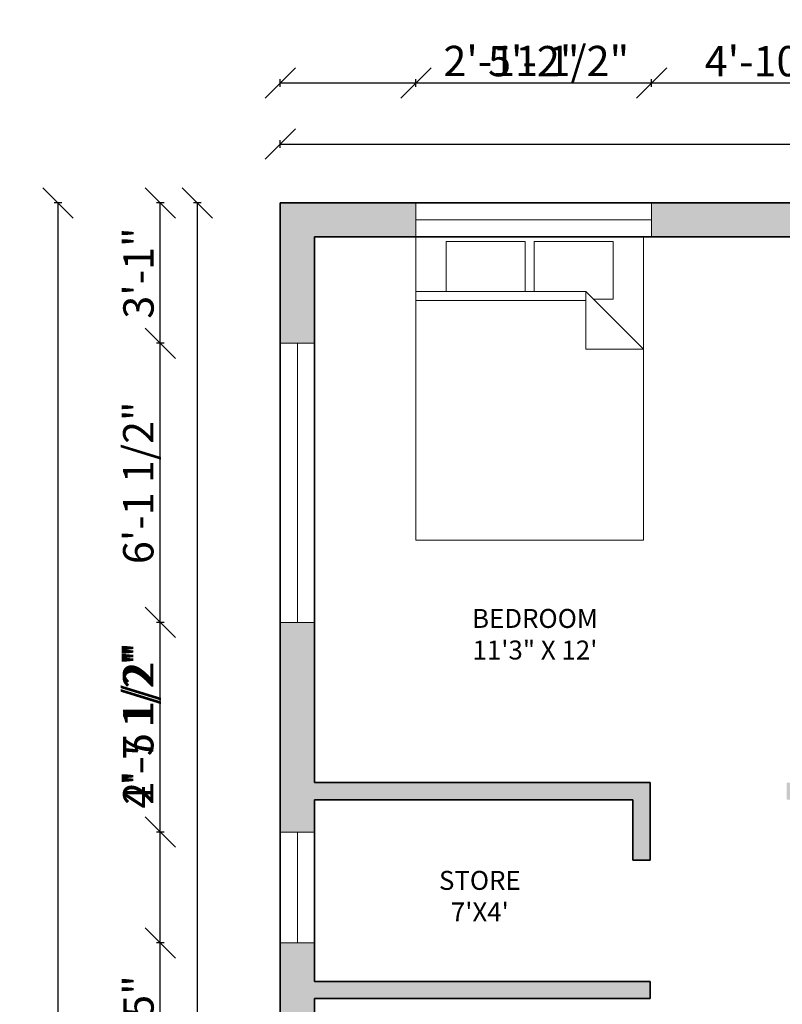
# Model space of a CAD drawing. Units: inches. Extents: x 2561 to 3163, y 493 to 1211.
# Tile 7 of 8: x 2561 to 2762, y 882 to 1141. Entities that reach past the tile are written whole.
import ezdxf

# ---------------------------------------------------------------- set-up
doc = ezdxf.new("R2010")
doc.units = ezdxf.units.IN
for name, color, linetype, lineweight in [('A-ANNO-DIMS', 2, 'Continuous', 18), ('A-AREA-IDEN', 7, 'Continuous', 18), ('A-FURN', 8, 'Continuous', 18), ('A-GLAZ', 4, 'Continuous', 18), ('A-WALL', 7, 'Continuous', 35), ('A-WALL-PATT', 24, 'Continuous', 13)]:
    doc.layers.add(name, color=color, linetype=linetype, lineweight=lineweight)
doc.styles.get("Standard").update_dxf_attribs({"font": 'arial.ttf'})
doc.dimstyles.new('ISO-25', dxfattribs={"dimtxt": 8, "dimasz": 8, "dimexe": 1, "dimexo": 1, "dimtad": 1, "dimlunit": 3, "dimtxsty": 'Standard', "dimblk": 'OBLIQUE', "dimcen": 2.5, "dimadec": 0, "dimazin": 0, "dimtfac": 1, "dimtmove": 0, "dimatfit": 3, "dimfxl": 1, "dimfxlon": 1, "dimarcsym": 0})

# ---------------------------------------------------------------- blocks, each defined once
blk = doc.blocks.new('Bed - Queen')
for p, q in [((0, -80.00003), (0, 0)), ((0, 0), (59.99999, 0)), ((59.99999, 0), (59.99999, -80.00003)), ((7.99999, -1.2), (28.79998, -1.2)), ((7.99999, -14.4), (7.99999, -1.2)), ((28.79998, -1.2), (28.79998, -14.4)), ((31.19999, -1.2), (51.99999, -1.2)), ((31.19999, -14.4), (31.19999, -1.2)), ((51.99999, -1.2), (51.99999, -16.4)), ((0, -14.4), (44.8, -14.4)), ((59.99999, -29.6), (44.8, -14.4)), ((44.8, -14.4), (44.8, -29.6)), ((44.8, -16.8), (0, -16.8)), ((51.99999, -16.4), (46.79936, -16.4)), ((44.8, -29.6), (59.99999, -29.6)), ((59.99999, -80.00003), (0, -80.00003))]:
    blk.add_line(p, q)
blk = doc.blocks.new('_Oblique')
at = {"color": 0, "linetype": 'ByBlock', "lineweight": -2}
blk.add_line((-0.5, -0.5), (0.5, 0.5), dxfattribs=at)
blk = doc.blocks.new('*D8')
at = {"layer": 'A-ANNO-DIMS', "color": 0, "lineweight": -2, "transparency": 16777216}
for p, q in [((2629.27, 1107.6), (2629.27, 1109.6)), ((3109.27, 1107.6), (3109.27, 1109.6)), ((2629.27, 1108.6), (3109.27, 1108.6))]:
    blk.add_line(p, q, dxfattribs=at)
at = {"layer": 'Defpoints', "color": 0, "transparency": 16777216}
for p in [(3109.27, 1108.6), (2629.27, 1093.07), (3109.27, 1093.07)]:
    blk.add_point(p, dxfattribs=at)
at = {"layer": 'A-ANNO-DIMS', "color": 0, "lineweight": -2, "transparency": 16777216, "xscale": 8, "yscale": 8, "zscale": 8, "rotation": 180}
blk.add_blockref('_Oblique', (2629.27, 1108.6), dxfattribs=at)
at = {"layer": 'A-ANNO-DIMS', "color": 0, "lineweight": -2, "transparency": 16777216, "xscale": 8, "yscale": 8, "zscale": 8}
blk.add_blockref('_Oblique', (3109.27, 1108.6), dxfattribs=at)
at = {"layer": 'A-ANNO-DIMS', "color": 0, "transparency": 16777216, "insert": (2869.27, 1113.31), "char_height": 8, "attachment_point": 5}
blk.add_mtext("40'", dxfattribs=at)
blk = doc.blocks.new('*D16')
at = {"layer": 'A-ANNO-DIMS', "color": 0, "lineweight": -2, "transparency": 16777216}
for p, q in [((2608.39, 1093.07), (2606.39, 1093.07)), ((2607.39, 1093.07), (2607.39, 614.57)), ((2608.39, 614.57), (2606.39, 614.57))]:
    blk.add_line(p, q, dxfattribs=at)
at = {"layer": 'Defpoints', "color": 0, "transparency": 16777216}
for p in [(2629.27, 1093.07), (2607.39, 614.57), (2629.27, 614.57)]:
    blk.add_point(p, dxfattribs=at)
at = {"layer": 'A-ANNO-DIMS', "color": 0, "lineweight": -2, "transparency": 16777216, "xscale": 8, "yscale": 8, "zscale": 8}
for p, rotation in [((2607.39, 1093.07), 90), ((2607.39, 614.57), 270)]:
    blk.add_blockref('_Oblique', p, dxfattribs=dict(at, rotation=rotation))
at = {"layer": 'A-ANNO-DIMS', "color": 0, "transparency": 16777216, "insert": (2602.67, 853.82), "char_height": 8, "attachment_point": 5, "rotation": 90}
blk.add_mtext('39\'-10.5"', dxfattribs=at)
blk = doc.blocks.new('*D17')
at = {"layer": 'A-ANNO-DIMS', "color": 0, "lineweight": -2, "transparency": 16777216}
for p, q in [((2571.63, 1093.07), (2569.63, 1093.07)), ((2570.63, 1093.07), (2570.63, 529.07)), ((2571.63, 529.07), (2569.63, 529.07))]:
    blk.add_line(p, q, dxfattribs=at)
at = {"layer": 'Defpoints', "color": 0, "transparency": 16777216}
for p in [(2629.27, 1093.07), (2570.63, 529.07), (3109.27, 529.07)]:
    blk.add_point(p, dxfattribs=at)
at = {"layer": 'A-ANNO-DIMS', "color": 0, "lineweight": -2, "transparency": 16777216, "xscale": 8, "yscale": 8, "zscale": 8}
for p, rotation in [((2570.63, 1093.07), 90), ((2570.63, 529.07), 270)]:
    blk.add_blockref('_Oblique', p, dxfattribs=dict(at, rotation=rotation))
at = {"layer": 'A-ANNO-DIMS', "color": 0, "transparency": 16777216, "insert": (2566, 811.07), "char_height": 8, "attachment_point": 5, "rotation": 90}
blk.add_mtext("47'", dxfattribs=at)
blk = doc.blocks.new('*D33')
at = {"layer": 'A-ANNO-DIMS', "color": 0, "lineweight": -2, "transparency": 16777216}
for p, q in [((2629.27, 1123.72), (2629.27, 1125.72)), ((2665.02, 1123.72), (2665.02, 1125.72)), ((2629.27, 1124.72), (2665.02, 1124.72)), ((2665.02, 1124.72), (2720.53, 1124.72))]:
    blk.add_line(p, q, dxfattribs=at)
at = {"layer": 'Defpoints', "color": 0, "transparency": 16777216}
for p in [(2665.02, 1124.72), (2629.27, 1093.07), (2665.02, 1093.07)]:
    blk.add_point(p, dxfattribs=at)
at = {"layer": 'A-ANNO-DIMS', "color": 0, "lineweight": -2, "transparency": 16777216, "xscale": 8, "yscale": 8, "zscale": 8, "rotation": 180}
blk.add_blockref('_Oblique', (2629.27, 1124.72), dxfattribs=at)
at = {"layer": 'A-ANNO-DIMS', "color": 0, "lineweight": -2, "transparency": 16777216, "xscale": 8, "yscale": 8, "zscale": 8}
blk.add_blockref('_Oblique', (2665.02, 1124.72), dxfattribs=at)
at = {"layer": 'A-ANNO-DIMS', "color": 0, "transparency": 16777216, "insert": (2696.78, 1129.48), "char_height": 8, "attachment_point": 5}
blk.add_mtext('2\'-11 1/2"', dxfattribs=at)
blk = doc.blocks.new('*D34')
at = {"layer": 'A-ANNO-DIMS', "color": 0, "lineweight": -2, "transparency": 16777216}
for p, q in [((2665.02, 1123.72), (2665.02, 1125.72)), ((2727.19, 1123.72), (2727.19, 1125.72)), ((2665.02, 1124.72), (2727.19, 1124.72))]:
    blk.add_line(p, q, dxfattribs=at)
at = {"layer": 'Defpoints', "color": 0, "transparency": 16777216}
for p in [(2727.19, 1124.72), (2665.02, 1093.07), (2727.19, 1093.07)]:
    blk.add_point(p, dxfattribs=at)
at = {"layer": 'A-ANNO-DIMS', "color": 0, "lineweight": -2, "transparency": 16777216, "xscale": 8, "yscale": 8, "zscale": 8, "rotation": 180}
blk.add_blockref('_Oblique', (2665.02, 1124.72), dxfattribs=at)
at = {"layer": 'A-ANNO-DIMS', "color": 0, "lineweight": -2, "transparency": 16777216, "xscale": 8, "yscale": 8, "zscale": 8}
blk.add_blockref('_Oblique', (2727.19, 1124.72), dxfattribs=at)
at = {"layer": 'A-ANNO-DIMS', "color": 0, "transparency": 16777216, "insert": (2696.11, 1129.43), "char_height": 8, "attachment_point": 5}
blk.add_mtext('5\'-2"', dxfattribs=at)
blk = doc.blocks.new('*D35')
at = {"layer": 'A-ANNO-DIMS', "color": 0, "lineweight": -2, "transparency": 16777216}
for p, q in [((2727.19, 1123.72), (2727.19, 1125.72)), ((2785.37, 1123.72), (2785.37, 1125.72)), ((2727.19, 1124.72), (2785.37, 1124.72))]:
    blk.add_line(p, q, dxfattribs=at)
at = {"layer": 'Defpoints', "color": 0, "transparency": 16777216}
for p in [(2785.37, 1124.72), (2727.19, 1093.07), (2785.37, 1093.07)]:
    blk.add_point(p, dxfattribs=at)
at = {"layer": 'A-ANNO-DIMS', "color": 0, "lineweight": -2, "transparency": 16777216, "xscale": 8, "yscale": 8, "zscale": 8, "rotation": 180}
blk.add_blockref('_Oblique', (2727.19, 1124.72), dxfattribs=at)
at = {"layer": 'A-ANNO-DIMS', "color": 0, "lineweight": -2, "transparency": 16777216, "xscale": 8, "yscale": 8, "zscale": 8}
blk.add_blockref('_Oblique', (2785.37, 1124.72), dxfattribs=at)
at = {"layer": 'A-ANNO-DIMS', "color": 0, "transparency": 16777216, "insert": (2756.28, 1129.43), "char_height": 8, "attachment_point": 5}
blk.add_mtext('4\'-10"', dxfattribs=at)
blk = doc.blocks.new('*D42')
at = {"layer": 'A-ANNO-DIMS', "color": 0, "lineweight": -2, "transparency": 16777216}
for p, q in [((2598.62, 1093.07), (2596.62, 1093.07)), ((2597.62, 1056.03), (2597.62, 1093.07)), ((2598.62, 1056.03), (2596.62, 1056.03))]:
    blk.add_line(p, q, dxfattribs=at)
at = {"layer": 'Defpoints', "color": 0, "transparency": 16777216}
for p in [(2597.62, 1093.07), (2629.27, 1093.07), (2629.27, 1056.03)]:
    blk.add_point(p, dxfattribs=at)
at = {"layer": 'A-ANNO-DIMS', "color": 0, "lineweight": -2, "transparency": 16777216, "xscale": 8, "yscale": 8, "zscale": 8}
for p, rotation in [((2597.62, 1093.07), 90), ((2597.62, 1056.03), 270)]:
    blk.add_blockref('_Oblique', p, dxfattribs=dict(at, rotation=rotation))
at = {"layer": 'A-ANNO-DIMS', "color": 0, "transparency": 16777216, "insert": (2592.91, 1074.55), "char_height": 8, "attachment_point": 5, "rotation": 90}
blk.add_mtext('3\'-1"', dxfattribs=at)
blk = doc.blocks.new('*D43')
at = {"layer": 'A-ANNO-DIMS', "color": 0, "lineweight": -2, "transparency": 16777216}
for p, q in [((2598.62, 1056.03), (2596.62, 1056.03)), ((2597.62, 982.37), (2597.62, 1056.03)), ((2598.62, 982.37), (2596.62, 982.37))]:
    blk.add_line(p, q, dxfattribs=at)
at = {"layer": 'Defpoints', "color": 0, "transparency": 16777216}
for p in [(2597.62, 1056.03), (2629.27, 1056.03), (2629.27, 982.37)]:
    blk.add_point(p, dxfattribs=at)
at = {"layer": 'A-ANNO-DIMS', "color": 0, "lineweight": -2, "transparency": 16777216, "xscale": 8, "yscale": 8, "zscale": 8}
for p, rotation in [((2597.62, 1056.03), 90), ((2597.62, 982.37), 270)]:
    blk.add_blockref('_Oblique', p, dxfattribs=dict(at, rotation=rotation))
at = {"layer": 'A-ANNO-DIMS', "color": 0, "transparency": 16777216, "insert": (2592.86, 1019.2), "char_height": 8, "attachment_point": 5, "rotation": 90}
blk.add_mtext('6\'-1 1/2"', dxfattribs=at)
blk = doc.blocks.new('*D44')
at = {"layer": 'A-ANNO-DIMS', "color": 0, "lineweight": -2, "transparency": 16777216}
for p, q in [((2598.62, 982.37), (2596.62, 982.37)), ((2597.62, 927.03), (2597.62, 982.37)), ((2598.62, 927.03), (2596.62, 927.03))]:
    blk.add_line(p, q, dxfattribs=at)
at = {"layer": 'Defpoints', "color": 0, "transparency": 16777216}
for p in [(2597.62, 982.37), (2629.27, 982.37), (2629.27, 927.03)]:
    blk.add_point(p, dxfattribs=at)
at = {"layer": 'A-ANNO-DIMS', "color": 0, "lineweight": -2, "transparency": 16777216, "xscale": 8, "yscale": 8, "zscale": 8}
for p, rotation in [((2597.62, 982.37), 90), ((2597.62, 927.03), 270)]:
    blk.add_blockref('_Oblique', p, dxfattribs=dict(at, rotation=rotation))
at = {"layer": 'A-ANNO-DIMS', "color": 0, "transparency": 16777216, "insert": (2592.86, 954.7), "char_height": 8, "attachment_point": 5, "rotation": 90}
blk.add_mtext('4\'-7 1/2"', dxfattribs=at)
blk = doc.blocks.new('*D45')
at = {"layer": 'A-ANNO-DIMS', "color": 0, "lineweight": -2, "transparency": 16777216}
for p, q in [((2597.62, 927.03), (2597.62, 976.32)), ((2598.62, 927.03), (2596.62, 927.03)), ((2597.62, 897.75), (2597.62, 927.03)), ((2598.62, 897.75), (2596.62, 897.75))]:
    blk.add_line(p, q, dxfattribs=at)
at = {"layer": 'Defpoints', "color": 0, "transparency": 16777216}
for p in [(2597.62, 927.03), (2629.27, 927.03), (2629.27, 897.75)]:
    blk.add_point(p, dxfattribs=at)
at = {"layer": 'A-ANNO-DIMS', "color": 0, "lineweight": -2, "transparency": 16777216, "xscale": 8, "yscale": 8, "zscale": 8}
for p, rotation in [((2597.62, 927.03), 90), ((2597.62, 897.75), 270)]:
    blk.add_blockref('_Oblique', p, dxfattribs=dict(at, rotation=rotation))
at = {"layer": 'A-ANNO-DIMS', "color": 0, "transparency": 16777216, "insert": (2592.86, 955.67), "char_height": 8, "attachment_point": 5, "rotation": 90}
blk.add_mtext('2\'-5 1/2"', dxfattribs=at)
blk = doc.blocks.new('*D46')
at = {"layer": 'A-ANNO-DIMS', "color": 0, "lineweight": -2, "transparency": 16777216}
for p, q in [((2598.62, 897.75), (2596.62, 897.75)), ((2597.62, 856.59), (2597.62, 897.75)), ((2598.62, 856.59), (2596.62, 856.59))]:
    blk.add_line(p, q, dxfattribs=at)
at = {"layer": 'Defpoints', "color": 0, "transparency": 16777216}
for p in [(2597.62, 897.75), (2629.27, 897.75), (2629.27, 856.59)]:
    blk.add_point(p, dxfattribs=at)
at = {"layer": 'A-ANNO-DIMS', "color": 0, "lineweight": -2, "transparency": 16777216, "xscale": 8, "yscale": 8, "zscale": 8}
for p, rotation in [((2597.62, 897.75), 90), ((2597.62, 856.59), 270)]:
    blk.add_blockref('_Oblique', p, dxfattribs=dict(at, rotation=rotation))
at = {"layer": 'A-ANNO-DIMS', "color": 0, "transparency": 16777216, "insert": (2592.91, 877.17), "char_height": 8, "attachment_point": 5, "rotation": 90}
blk.add_mtext('3\'-5"', dxfattribs=at)

msp = doc.modelspace()

# ---------------------------------------------------------------- hatches: boundary and pattern name
at = {"layer": 'A-WALL-PATT'}
h = msp.add_hatch(color=256, dxfattribs=at)
h.dxf.hatch_style = 1
h.paths.add_polyline_path([(2665.022, 1093.069), (2629.274, 1093.069), (2629.274, 1056.034), (2638.274, 1056.034), (2638.274, 1084.069), (2665.022, 1084.069)])
h.paths.add_polyline_path([(2785.37, 1093.069), (2727.193, 1093.069), (2727.193, 1084.069), (2773.274, 1084.069), (2773.274, 940.069), (2762.774, 940.069), (2762.774, 935.569), (2777.774, 935.569), (2777.774, 971.569), (2825.774, 971.569), (2825.774, 935.569), (2921.774, 935.569), (2921.774, 940.069), (2830.274, 940.069), (2830.274, 976.069), (2777.774, 976.069), (2777.774, 1084.069), (2785.37, 1084.069)])
h.paths.add_polyline_path([(2856.568, 1093.069), (2816.168, 1093.069), (2816.168, 1084.069), (2825.774, 1084.069), (2825.774, 1008.069), (2830.274, 1008.069), (2830.274, 1084.069), (2856.568, 1084.069)], flags=17)
h.paths.add_polyline_path([(3006.866, 1093.069), (2929.24, 1093.069), (2929.24, 1084.069), (2962.274, 1084.069), (2962.274, 940.069), (2957.774, 940.069), (2957.774, 935.569), (2970.774, 935.569), (2970.774, 940.069), (2968.274, 940.069), (2968.274, 1084.069), (3006.866, 1084.069)])
h.paths.add_polyline_path([(3109.274, 1093.069), (3068.804, 1093.069), (3068.804, 1084.069), (3100.274, 1084.069), (3100.274, 1061.194), (3109.274, 1061.194)])
h.paths.add_polyline_path([(3109.274, 991.723), (3100.274, 991.723), (3100.274, 940.069), (3010.774, 940.069), (3010.774, 935.569), (3010.774, 911.569), (3015.274, 911.569), (3015.274, 935.569), (3100.274, 935.569), (3100.274, 927.07), (3109.274, 927.07)])
h.paths.add_polyline_path([(3109.274, 897.327), (3100.274, 897.327), (3100.274, 881.569), (2957.774, 881.569), (2957.774, 872.569), (3100.274, 872.569), (3100.274, 805.791), (3109.274, 805.791)])
h.paths.add_polyline_path([(2638.274, 982.372), (2629.274, 982.372), (2629.274, 927.027), (2638.274, 927.027), (2638.274, 935.569), (2722.274, 935.569), (2722.274, 919.569), (2726.774, 919.569), (2726.774, 940.069), (2638.274, 940.069)])
h.paths.add_polyline_path([(2638.274, 883.069), (2726.774, 883.069), (2726.774, 887.569), (2638.274, 887.569), (2638.274, 897.75), (2629.274, 897.75), (2629.274, 856.591), (2638.274, 856.591)])
h.paths.add_polyline_path([(2726.774, 851.069), (2722.274, 851.069), (2722.274, 772.069), (2638.274, 772.069), (2638.274, 802.178), (2629.274, 802.178), (2629.274, 725.136), (2638.274, 725.136), (2638.274, 767.569), (2726.774, 767.569)])
h.paths.add_polyline_path([(2638.274, 659.235), (2629.274, 659.235), (2629.274, 614.569), (2638.274, 614.569)])
h.paths.add_polyline_path([(2664.613, 623.569), (2638.274, 623.569), (2638.274, 614.569), (2664.613, 614.569)])
h.paths.add_polyline_path([(2787.908, 623.569), (2777.774, 623.569), (2777.774, 767.569), (2825.774, 767.569), (2825.774, 659.569), (2830.274, 659.569), (2830.274, 767.569), (2836.774, 767.569), (2836.774, 772.069), (2766.674, 772.069), (2766.674, 767.569), (2773.274, 767.569), (2773.274, 623.569), (2722.435, 623.569), (2722.435, 614.569), (2787.908, 614.569)])
h.paths.add_polyline_path([(2883.664, 623.569), (2867.474, 623.569), (2818.294, 623.569), (2818.294, 614.569), (2883.664, 614.569)])
h.paths.add_polyline_path([(2965.274, 772.069), (2872.774, 772.069), (2872.774, 767.569), (2962.274, 767.569), (2962.274, 623.569), (2936.565, 623.569), (2936.565, 614.569), (2965.274, 614.569)])
h.paths.add_polyline_path([(3109.274, 758.846), (3100.274, 758.846), (3100.274, 701.069), (3013.274, 701.069), (3013.274, 695.069), (3109.274, 695.069)])
h.paths.add_polyline_path([(2965.274, 824.569), (2957.774, 824.569), (2957.774, 772.069), (2965.274, 772.069)])

# ---------------------------------------------------------------- linework, layer by layer
at = {"layer": 'A-GLAZ'}
for p, q in [((2665.022, 1093.069), (2665.022, 1084.069)), ((2727.193, 1093.069), (2727.193, 1084.069)), ((2638.274, 1056.034), (2629.274, 1056.034)), ((2638.274, 982.372), (2629.274, 982.372)), ((2638.274, 927.027), (2629.274, 927.027)), ((2638.274, 897.75), (2629.274, 897.75))]:
    msp.add_line(p, q, dxfattribs=at)
for points in [[(2727.193, 1088.569), (2665.022, 1088.569)], [(2633.774, 1056.034), (2633.774, 982.372)], [(2633.774, 927.027), (2633.774, 897.75)]]:
    msp.add_lwpolyline(points, dxfattribs=at)
at = {"layer": 'A-WALL'}
for p, q in [((2638.274, 1084.069), (2638.274, 940.069)), ((2773.274, 1084.069), (2638.274, 1084.069)), ((2726.774, 940.069), (2638.274, 940.069)), ((2726.774, 919.569), (2726.774, 940.069)), ((2638.274, 935.569), (2638.274, 887.569)), ((2722.274, 935.569), (2638.274, 935.569)), ((2722.274, 935.569), (2722.274, 919.569)), ((2722.274, 919.569), (2726.774, 919.569)), ((2726.774, 887.569), (2638.274, 887.569)), ((2726.774, 883.069), (2726.774, 887.569)), ((2638.274, 883.069), (2638.274, 772.069)), ((2638.274, 883.069), (2726.774, 883.069))]:
    msp.add_line(p, q, dxfattribs=at)
msp.add_lwpolyline([(3109.274, 695.069), (3109.274, 1093.069), (2629.274, 1093.069), (2629.274, 614.569), (2965.274, 614.569)], dxfattribs=at)

# ---------------------------------------------------------------- block references
at = {"layer": 'A-FURN'}
msp.add_blockref('Bed - Queen', (2665.022, 1084.069), dxfattribs=at)

# ---------------------------------------------------------------- texts
at = {"layer": 'A-AREA-IDEN', "char_height": 5, "attachment_point": 1}
for s, insert in [('\\pxqc;BEDROOM\\P11\'3" X 12\'', (2665.811, 985.897)), ("\\pxqc;STORE\\P7'X4'", (2651.276, 916.771))]:
    msp.add_mtext_dynamic_manual_height_columns(s, width=61.24894, gutter_width=12.5, heights=[0], dxfattribs=dict(at, insert=insert))

# ---------------------------------------------------------------- dimensions: what is measured, and where the dimension line sits
at = {"layer": 'A-ANNO-DIMS'}
for base, p1, p2, override, picture, middle in [((2665.022, 1124.719), (2629.274, 1093.069), (2665.022, 1093.069), {"dimdec": 1, "dimlfac": 1, "dimrnd": 0, "dimzin": 1, "dimdsep": 46, "dimlunit": 4, "dimfrac": 2}, '*D33', (2696.777, 1129.48)), ((2727.193, 1124.719), (2665.022, 1093.069), (2727.193, 1093.069), {"dimdec": 1, "dimlfac": 1, "dimrnd": 0, "dimzin": 1, "dimdsep": 46, "dimlunit": 4, "dimfrac": 2}, '*D34', (2696.107, 1129.428)), ((2785.37, 1124.719), (2727.193, 1093.069), (2785.37, 1093.069), {"dimdec": 1, "dimlfac": 1, "dimrnd": 0, "dimzin": 1, "dimdsep": 46, "dimlunit": 4, "dimfrac": 2}, '*D35', (2756.281, 1129.428)), ((3109.274, 1108.596), (2629.274, 1093.069), (3109.274, 1093.069), {"dimclrd": 0, "dimclre": 0, "dimclrt": 0}, '*D8', (2869.274, 1113.305))]:
    dim = msp.add_linear_dim(base=base, p1=p1, p2=p2, dimstyle='ISO-25', override=override, dxfattribs=at)
    dim.commit()
    dim.dimension.update_dxf_attribs({"geometry": picture, "text_midpoint": middle})
for base, p1, p2, override, picture, middle in [((2570.627, 529.069), (2629.274, 1093.069), (3109.274, 529.069), {"dimclrd": 0, "dimclre": 0, "dimclrt": 0}, '*D17', (2566.002, 811.069)), ((2597.624, 1093.069), (2629.274, 1056.034), (2629.274, 1093.069), {"dimdec": 1, "dimlfac": 1, "dimrnd": 0, "dimzin": 1, "dimdsep": 46, "dimlunit": 4, "dimfrac": 2}, '*D42', (2592.911, 1074.551)), ((2607.386, 614.569), (2629.274, 1093.069), (2629.274, 614.569), {"dimclrd": 0, "dimclre": 0, "dimclrt": 0}, '*D16', (2602.674, 853.819)), ((2597.624, 1056.034), (2629.274, 982.372), (2629.274, 1056.034), {"dimdec": 1, "dimlfac": 1, "dimrnd": 0, "dimzin": 1, "dimdsep": 46, "dimlunit": 4, "dimfrac": 2}, '*D43', (2592.862, 1019.203)), ((2597.624, 982.372), (2629.274, 927.027), (2629.274, 982.372), {"dimdec": 1, "dimlfac": 1, "dimrnd": 0, "dimzin": 1, "dimdsep": 46, "dimlunit": 4, "dimfrac": 2}, '*D44', (2592.862, 954.7)), ((2597.624, 927.027), (2629.274, 897.75), (2629.274, 927.027), {"dimdec": 1, "dimlfac": 1, "dimrnd": 0, "dimzin": 1, "dimdsep": 46, "dimlunit": 4, "dimfrac": 2}, '*D45', (2592.862, 955.674)), ((2597.624, 897.75), (2629.274, 856.591), (2629.274, 897.75), {"dimdec": 1, "dimlfac": 1, "dimrnd": 0, "dimzin": 1, "dimdsep": 46, "dimlunit": 4, "dimfrac": 2}, '*D46', (2592.911, 877.171))]:
    dim = msp.add_linear_dim(base=base, p1=p1, p2=p2, angle=90, dimstyle='ISO-25', override=override, dxfattribs=at)
    dim.commit()
    dim.dimension.update_dxf_attribs({"geometry": picture, "text_midpoint": middle})

doc.saveas('drawing.dxf')
